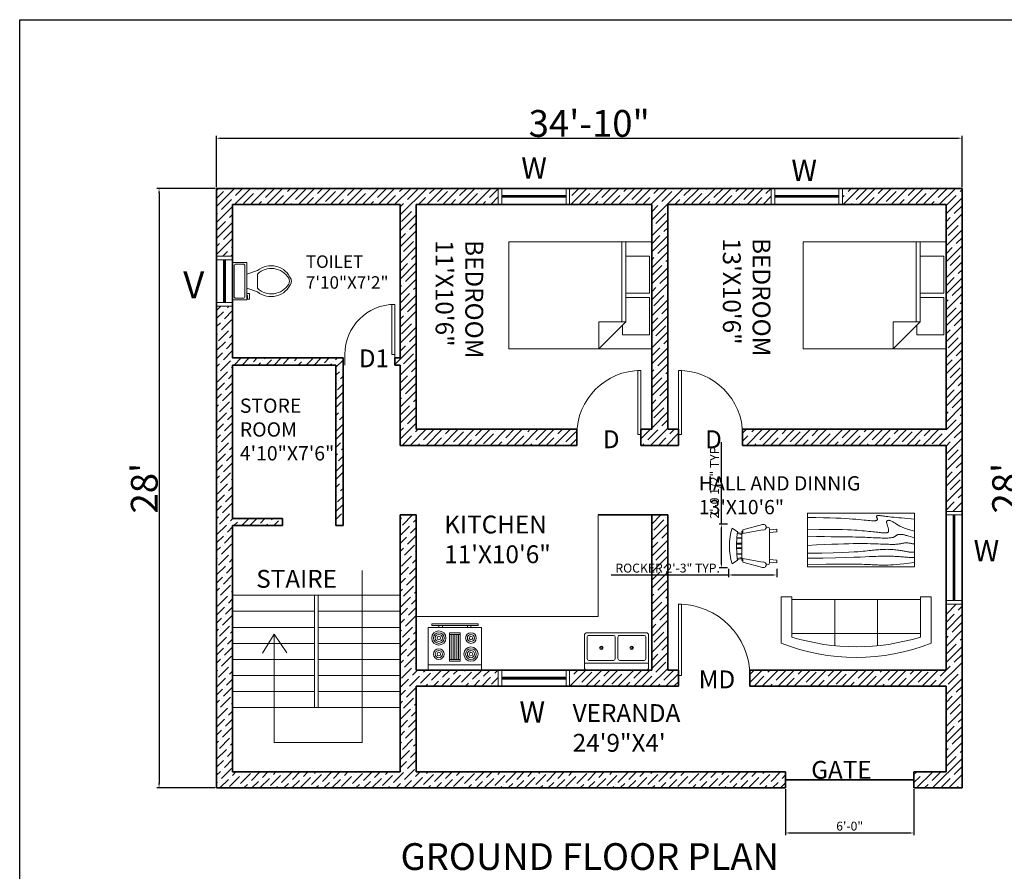
# Model space of a CAD drawing. Units: inches. Extents: x 1662 to 23131, y 1265 to 19127.
# Tile 12 of 26: x 17165 to 17717, y 8255 to 8732. Entities that reach past the tile are written whole.
import ezdxf

# ---------------------------------------------------------------- set-up
doc = ezdxf.new("R2010")
doc.units = ezdxf.units.IN
for name, color, linetype, lineweight in [('A-ANNO-DIMS', 4, 'Continuous', 18), ('A-ANNO-IDEN', 7, 'Continuous', 18), ('A-ANNO-TITL', 7, 'Continuous', 35), ('A-ANNO-TTLB', 7, 'Continuous', 25), ('A-AREA-IDEN', 7, 'Continuous', 18), ('A-DOOR', 3, 'Continuous', 18), ('A-EQPM', 8, 'Continuous', 18), ('A-FLOR-CASE', 8, 'Continuous', 18), ('A-FLOR-FIXT', 9, 'Continuous', 18), ('A-FLOR-STRS', 7, 'Continuous', 18), ('A-FURN', 8, 'Continuous', 18), ('A-GLAZ', 4, 'Continuous', 18), ('A-WALL', 7, 'Continuous', 35), ('A-WALL-PATT', 8, 'Continuous', 13)]:
    doc.layers.add(name, color=color, linetype=linetype, lineweight=lineweight)
doc.styles.get("Standard").update_dxf_attribs({"font": 'arial.ttf'})
doc.dimstyles.new('ISO-25', dxfattribs={"dimtxt": 5, "dimasz": 2.5, "dimexe": 1.25, "dimexo": 0.625, "dimtad": 1, "dimlunit": 3, "dimtxsty": 'Standard', "dimcen": 2.5, "dimadec": 0, "dimazin": 0, "dimtfac": 1, "dimtmove": 0, "dimatfit": 3, "dimfxl": 1, "dimarcsym": 0})

# ---------------------------------------------------------------- blocks, each defined once
blk = doc.blocks.new('*D63')
at = {"layer": 'A-ANNO-DIMS', "color": 0, "lineweight": -2, "transparency": 16777216}
for p, q in [((17275.26, 8638.02), (17275.26, 8666.76)), ((17693.26, 8638.02), (17693.26, 8666.76)), ((17277.76, 8665.51), (17690.76, 8665.51))]:
    blk.add_line(p, q, dxfattribs=at)
at = {"layer": 'A-ANNO-DIMS', "color": 0, "transparency": 16777216}
for points in [[(17277.76, 8665.93), (17277.76, 8665.09), (17275.26, 8665.51)], [(17690.76, 8665.93), (17690.76, 8665.09), (17693.26, 8665.51)]]:
    blk.add_solid(points, dxfattribs=at)
at = {"layer": 'Defpoints', "color": 0, "transparency": 16777216}
for p in [(17693.26, 8665.51), (17275.26, 8637.39), (17693.26, 8637.39)]:
    blk.add_point(p, dxfattribs=at)
at = {"layer": 'A-ANNO-DIMS', "color": 0, "transparency": 16777216, "insert": (17484.26, 8673.8), "char_height": 5, "attachment_point": 5}
blk.add_mtext('{\\H3x;34\'-10"}', dxfattribs=at)
blk = doc.blocks.new('*D64')
at = {"layer": 'A-ANNO-DIMS', "color": 0, "lineweight": -2, "transparency": 16777216}
for p, q in [((17274.63, 8637.39), (17241.85, 8637.39)), ((17243.1, 8634.89), (17243.1, 8303.89)), ((17274.63, 8301.39), (17241.85, 8301.39))]:
    blk.add_line(p, q, dxfattribs=at)
at = {"layer": 'A-ANNO-DIMS', "color": 0, "transparency": 16777216}
for points in [[(17242.68, 8634.89), (17243.51, 8634.89), (17243.1, 8637.39)], [(17242.68, 8303.89), (17243.51, 8303.89), (17243.1, 8301.39)]]:
    blk.add_solid(points, dxfattribs=at)
at = {"layer": 'Defpoints', "color": 0, "transparency": 16777216}
for p in [(17275.26, 8637.39), (17243.1, 8301.39), (17275.26, 8301.39)]:
    blk.add_point(p, dxfattribs=at)
at = {"layer": 'A-ANNO-DIMS', "color": 0, "transparency": 16777216, "insert": (17234.81, 8469.39), "char_height": 5, "attachment_point": 5, "rotation": 90}
blk.add_mtext("{\\H3x;28'}", dxfattribs=at)
blk = doc.blocks.new('*U10')
for p, q in [((0, 0), (0, -6)), ((40, 0), (40, -6))]:
    blk.add_line(p, q)
blk.add_lwpolyline([(0, 0), (0, 40), (1.75, 40), (1.75, 0)], close=True)
blk.add_arc((0, 0), 40, 0, 90)
blk = doc.blocks.new('*U67')
for p, q in [((0, 0), (0, -6)), ((36, 0), (36, -6))]:
    blk.add_line(p, q)
blk.add_lwpolyline([(0, 0), (0, 36), (1.75, 36), (1.75, 0)], close=True)
blk.add_arc((0, 0), 36, 0, 90)
blk = doc.blocks.new('*U34')
for p, q in [((0, 0), (0, -6)), ((-36, 0), (-36, -6))]:
    blk.add_line(p, q)
blk.add_lwpolyline([(0, 0), (0, 36), (-1.75, 36), (-1.75, 0)], close=True)
blk.add_arc((0, 0), 36, 90, 180)
blk = doc.blocks.new('*U68')
for p, q in [((-28, 0), (-28, -6)), ((0, 0), (0, -6))]:
    blk.add_line(p, q)
blk.add_lwpolyline([(0, 0), (0, 28), (-1.75, 28), (-1.75, 0)], close=True)
blk.add_arc((0, 0), 28, 90, 180)
blk = doc.blocks.new('Bed - Queen')
for p, q in [((0, -80.00003), (0, 0)), ((0, 0), (59.99999, 0)), ((59.99999, 0), (59.99999, -80.00003)), ((7.99999, -1.2), (28.79998, -1.2)), ((7.99999, -14.4), (7.99999, -1.2)), ((28.79998, -1.2), (28.79998, -14.4)), ((31.19999, -1.2), (51.99999, -1.2)), ((31.19999, -14.4), (31.19999, -1.2)), ((51.99999, -1.2), (51.99999, -16.4)), ((0, -14.4), (44.8, -14.4)), ((59.99999, -29.6), (44.8, -14.4)), ((44.8, -14.4), (44.8, -29.6)), ((51.99999, -16.4), (46.79936, -16.4)), ((44.8, -16.8), (0, -16.8)), ((44.8, -29.6), (59.99999, -29.6)), ((59.99999, -80.00003), (0, -80.00003))]:
    blk.add_line(p, q)
blk = doc.blocks.new('Toilet - top')
for p, q in [((9.5, -6), (9.5, -2)), ((-10, -8.5), (-8, -8.5)), ((-10, -9.5), (-10, -8.5)), ((-7, -9.5), (-10, -9.5)), ((-8, -8.5), (-8, -8)), ((-7, -8), (-7, -9.5)), ((-4, -8), (-6, -14)), ((4, -8), (6, -14)), ((4, -14), (-4, -14))]:
    blk.add_line(p, q)
blk.add_lwpolyline([(10.5, -8), (10.5, 0), (-10.5, 0), (-10.5, -8)], close=True)
for points in [[(-9.5, -2), (-9.5, -6)], [(8.5, -1), (-8.5, -1)], [(-8.5, -7), (8.5, -7)]]:
    blk.add_lwpolyline(points)
for centre, radius, start, end in [((-8.62, -1.88), 0.884, 81.8699, 188.1301), ((8.62, -1.88), 0.884, 351.8699, 98.1301), ((-8.62, -6.12), 0.884, 171.8699, 278.1301), ((8.62, -6.12), 0.884, 261.8699, 8.1301), ((3.52, -21.58), 12.17, 141.4691, 247.9714), ((4.2, -21.82), 11.33, 136.3677, 238.9468), ((-3.52, -21.58), 12.17, 292.0284, 38.5307), ((-4.2, -21.82), 11.33, 301.053, 43.6321), ((0, -27.88), 4, 245.7318, 294.2682), ((0, -29), 4, 254.8605, 285.1395)]:
    blk.add_arc(centre, radius, start, end)
blk = doc.blocks.new('Range-Oven - 30 in top')
for p, q in [((0, -3), (30, -3)), ((12, -6), (18, -6)), ((13, -20), (13, -6)), ((14, -6), (14, -20)), ((15, -20), (15, -6)), ((16, -6), (16, -20)), ((17, -20), (17, -6)), ((18, -20), (12, -20)), ((6, -24), (6, -25)), ((8, -25), (8, -24)), ((22, -25), (22, -24)), ((24, -24), (24, -25))]:
    blk.add_line(p, q)
for points in [[(0, -24), (0, 0), (30, 0), (30, -24)], [(12, -21), (12, -5), (18, -5), (18, -21)], [(2, -26), (2, -25), (28, -25), (28, -26)]]:
    blk.add_lwpolyline(points, close=True)
for centre, radius in [((6, -9), 4), ((6, -9), 3), ((6, -9), 2), ((6, -9), 1), ((24, -9), 3), ((24, -9), 2), ((24, -9), 1), ((6, -18), 3), ((6, -18), 2), ((24, -18), 4), ((24, -18), 3), ((24, -18), 2), ((6, -18), 1), ((24, -18), 1)]:
    blk.add_circle(centre, radius)
blk = doc.blocks.new('Sink-double - 36 in top')
for p, q in [((-18, -4), (18, -4)), ((-0.75, -18.5), (-0.75, -6.5)), ((0.75, -6.5), (0.75, -18.5))]:
    blk.add_line(p, q)
for points in [[(-16.5, 0), (16.5, 0)], [(-18, -19.5), (-18, -1.5)], [(-15.5, -5.5), (-1.75, -5.5)], [(1.75, -5.5), (15.5, -5.5)], [(18, -1.5), (18, -19.5)], [(-16.5, -18.5), (-16.5, -6.5)], [(16.5, -6.5), (16.5, -18.5)], [(16.5, -21), (-16.5, -21)], [(-1.75, -19.5), (-15.5, -19.5)], [(15.5, -19.5), (1.75, -19.5)]]:
    blk.add_lwpolyline(points)
for centre, radius in [((-8.5, -12.5), 1), ((-8.5, -12.5), 0.5), ((8.5, -12.5), 1), ((8.5, -12.5), 0.5)]:
    blk.add_circle(centre, radius)
for centre, radius, start, end in [((-16.5, -1.5), 1.5, 90, 180), ((16.5, -1.5), 1.5, 0, 90), ((-15.5, -6.5), 1, 90, 180), ((-1.75, -6.5), 1, 0, 90), ((1.75, -6.5), 1, 90, 180), ((15.5, -6.5), 1, 0, 90), ((-16.5, -19.5), 1.5, 180, 270), ((-15.5, -18.5), 1, 180, 270), ((-1.75, -18.5), 1, 270, 0), ((1.75, -18.5), 1, 180, 270), ((15.5, -18.5), 1, 270, 0), ((16.5, -19.5), 1.5, 270, 0)]:
    blk.add_arc(centre, radius, start, end)
blk = doc.blocks.new('Sofa - Roundback 7 ft.')
for p, q in [((-12.00002, -32.4421), (-12.00003, -6.5971)), ((11.99997, -32.4421), (11.99998, -6.5971)), ((-36.000027, -34), (-36.000027, -11.4696)), ((-35.999844, -13.3819), (35.9998, -13.3819)), ((35.99998, -34), (35.99998, -11.4696)), ((-36.000027, -32.4421), (35.99998, -32.4421))]:
    blk.add_line(p, q)
for points in [[(-36.000027, -34), (-42.000027, -34), (-42.000027, -8)], [(41.99998, -8), (41.99998, -34), (35.99998, -34)]]:
    blk.add_lwpolyline(points)
for centre, radius, start, end in [((0, -114.25), 114.25, 68.43141, 111.5686), ((-0.00001, -127.1968), 121.1968, 72.72033, 107.2797)]:
    blk.add_arc(centre, radius, start, end)
blk = doc.blocks.new('Table - Rectangular Woodgrain 60 x 30 in.')
for p, q in [((0, 0), (0, -30)), ((60, 0), (0, 0)), ((60, -30), (60, 0)), ((0, -30), (60, -30))]:
    blk.add_line(p, q)
for points in [[(0, -2.4), (4.8155, -2.418), (9.0302, -2.4688), (12.709, -2.5477), (15.9167, -2.65), (18.7181, -2.7711), (21.1781, -2.9063), (23.3616, -3.0508), (25.3333, -3.2), (27.1477, -3.3495), (28.8172, -3.4958), (30.3437, -3.636), (31.7291, -3.7667), (32.9756, -3.8849), (34.0849, -3.9875), (35.059, -4.0714), (35.9, -4.1334), (36.6114, -4.1711), (37.2041, -4.1854), (37.6906, -4.1779), (38.0833, -4.15), (38.3948, -4.1034), (38.6375, -4.0396), (38.8239, -3.9602), (38.9666, -3.8667), (39.0764, -3.7608), (39.1573, -3.6448), (39.2116, -3.521), (39.2416, -3.3917), (39.2498, -3.2593), (39.2385, -3.1261), (39.21, -2.9944), (39.1666, -2.8667), (39.111, -2.7447), (39.0468, -2.6281), (38.978, -2.5163), (38.9083, -2.4083), (38.8418, -2.3035), (38.7823, -2.201), (38.7337, -2.1001), (38.7, -2), (38.6844, -1.9003), (38.6875, -1.8021), (38.7094, -1.707), (38.75, -1.6167), (38.8094, -1.5326), (38.8875, -1.4563), (38.9844, -1.3893), (39.1, -1.3333), (39.2351, -1.2896), (39.3937, -1.2583), (39.5804, -1.2396), (39.8, -1.2333), (40.057, -1.2396), (40.3562, -1.2583), (40.7023, -1.2896), (41.1, -1.3333), (41.5547, -1.3895), (42.0755, -1.4573), (42.6721, -1.5361), (43.3542, -1.625), (44.1316, -1.7233), (45.014, -1.8302), (46.0114, -1.9449), (47.1333, -2.0667), (48.3862, -2.1947), (49.7625, -2.3281), (51.2513, -2.4663), (52.8416, -2.6083), (54.5226, -2.7535), (56.2833, -2.9011), (58.1127, -3.0501), (60, -3.2)], [(0, -9.2), (6.5759, -9.0858), (11.9385, -9.0365), (16.2527, -9.0418), (19.6833, -9.0917), (22.3952, -9.1759), (24.5531, -9.2844), (26.322, -9.4069), (27.8666, -9.5333), (29.3241, -9.6553), (30.7203, -9.7719), (32.0532, -9.8837), (33.3208, -9.9917), (34.5213, -10.0965), (35.6526, -10.199), (36.7128, -10.2999), (37.7, -10.4), (38.6129, -10.4996), (39.4531, -10.5969), (40.223, -10.6895), (40.925, -10.775), (41.5613, -10.8512), (42.1344, -10.9156), (42.6465, -10.966), (43.1, -11), (43.4976, -11.0158), (43.8437, -11.0136), (44.143, -10.9942), (44.4, -10.9583), (44.6195, -10.9069), (44.8062, -10.8406), (44.9648, -10.7603), (45.1, -10.6667), (45.2155, -10.5598), (45.3114, -10.4365), (45.3871, -10.2929), (45.4416, -10.125), (45.4743, -9.929), (45.4844, -9.7011), (45.4709, -9.4371), (45.4333, -9.1333), (45.3716, -8.7883), (45.2896, -8.4104), (45.1919, -8.0107), (45.0833, -7.6), (44.9685, -7.1893), (44.8521, -6.7896), (44.7388, -6.4117), (44.6333, -6.0667), (44.54, -5.7628), (44.4614, -5.4979), (44.4001, -5.2675), (44.3583, -5.0667), (44.3384, -4.8909), (44.3427, -4.7354), (44.3736, -4.5956), (44.4333, -4.4667), (44.5236, -4.3453), (44.6427, -4.2333), (44.7884, -4.1339), (44.9583, -4.05), (45.1501, -3.9849), (45.3614, -3.9417), (45.59, -3.9234), (45.8333, -3.9333), (46.0915, -3.9749), (46.3734, -4.0531), (46.6906, -4.1736), (47.0542, -4.3417), (47.4756, -4.5629), (47.9661, -4.8427), (48.5372, -5.1866), (49.2, -5.6), (49.9676, -6.0844), (50.8594, -6.625), (51.8965, -7.2031), (53.1, -7.8), (54.491, -8.3969), (56.0906, -8.975), (57.9199, -9.5156), (60, -10)], [(0, -12.8), (5.1847, -12.9322), (9.6213, -13.0323), (13.3963, -13.1059), (16.5958, -13.1583), (19.3063, -13.1952), (21.614, -13.2219), (23.6054, -13.2439), (25.3666, -13.2667), (26.9728, -13.2947), (28.4531, -13.3281), (29.8256, -13.3663), (31.1083, -13.4083), (32.3191, -13.4535), (33.476, -13.501), (34.597, -13.5501), (35.7, -13.6), (36.7984, -13.6497), (37.8875, -13.6979), (38.9578, -13.743), (40, -13.7833), (41.0047, -13.8174), (41.9625, -13.8438), (42.864, -13.8607), (43.7, -13.8667), (44.4631, -13.8604), (45.1552, -13.8417), (45.7801, -13.8104), (46.3416, -13.7667), (46.8439, -13.7104), (47.2906, -13.6417), (47.6858, -13.5604), (48.0333, -13.4667), (48.3375, -13.3608), (48.6042, -13.2448), (48.8396, -13.121), (49.05, -12.9917), (49.2417, -12.8593), (49.4208, -12.7261), (49.5937, -12.5944), (49.7667, -12.4667), (49.9452, -12.3451), (50.1323, -12.2313), (50.3303, -12.1268), (50.5416, -12.0333), (50.7686, -11.9524), (51.0135, -11.8854), (51.2788, -11.8341), (51.5666, -11.8), (51.8785, -11.7843), (52.2116, -11.7865), (52.562, -11.8059), (52.926, -11.8417), (53.2998, -11.8931), (53.6795, -11.9594), (54.0614, -12.0397), (54.4416, -12.1333), (54.8223, -12.2401), (55.2293, -12.3625), (55.6942, -12.5037), (56.2489, -12.6667), (56.9251, -12.8547), (57.7545, -13.0708), (58.7689, -13.3182), (60, -13.6)], [(0, -18), (5.124, -17.7273), (9.6609, -17.5057), (13.6705, -17.3303), (17.2125, -17.1958), (20.3467, -17.0973), (23.1328, -17.0297), (25.6307, -16.9878), (27.9, -16.9667), (29.9928, -16.9617), (31.9302, -16.9703), (33.7254, -16.9907), (35.3917, -17.0208), (36.9423, -17.0588), (38.3906, -17.1026), (39.7499, -17.1503), (41.0333, -17.2), (42.2519, -17.2496), (43.4073, -17.2969), (44.4986, -17.3395), (45.525, -17.375), (46.4858, -17.4012), (47.3802, -17.4156), (48.2074, -17.416), (48.9667, -17.4), (49.6583, -17.3662), (50.2872, -17.3167), (50.8595, -17.2547), (51.3812, -17.1833), (51.8584, -17.1057), (52.2971, -17.025), (52.7034, -16.9443), (53.0833, -16.8667), (53.443, -16.7951), (53.789, -16.7313), (54.128, -16.6768), (54.4666, -16.6334), (54.8115, -16.6024), (55.1693, -16.5854), (55.5465, -16.5841), (55.95, -16.6), (56.3828, -16.6337), (56.8346, -16.6823), (57.2915, -16.7418), (57.7396, -16.8084), (58.165, -16.878), (58.5539, -16.9469), (58.8924, -17.0111), (59.1666, -17.0667), (59.3679, -17.1107), (59.5078, -17.1438), (59.6032, -17.1675), (59.6708, -17.1833), (59.7275, -17.193), (59.7901, -17.1979), (59.8753, -17.1998), (60, -17.2)], [(0, -22.4), (8.0098, -22.2501), (14.4094, -22.1011), (19.4168, -21.9535), (23.25, -21.8083), (26.1269, -21.6663), (28.2656, -21.5281), (29.884, -21.3947), (31.2, -21.2667), (32.3967, -21.1448), (33.5172, -21.0292), (34.5697, -20.9198), (35.5625, -20.8167), (36.5037, -20.7198), (37.4015, -20.6292), (38.2642, -20.5448), (39.1, -20.4667), (39.9164, -20.3951), (40.7187, -20.3313), (41.5117, -20.2768), (42.3, -20.2333), (43.0883, -20.2024), (43.8812, -20.1854), (44.6836, -20.1841), (45.5, -20.2), (46.3328, -20.234), (47.1747, -20.2844), (48.0163, -20.3488), (48.8479, -20.425), (49.66, -20.5106), (50.4429, -20.6031), (51.1872, -20.7004), (51.8833, -20.8), (52.5246, -20.8999), (53.1166, -20.9995), (53.6681, -21.0983), (54.1875, -21.1958), (54.6834, -21.2919), (55.1646, -21.3859), (55.6394, -21.4777), (56.1167, -21.5667), (56.6028, -21.6515), (57.0961, -21.7266), (57.5929, -21.7852), (58.0896, -21.8208), (58.5823, -21.8268), (59.0674, -21.7964), (59.5412, -21.723), (60, -21.6)], [(0, -25.2), (8.6355, -25.0504), (15.7026, -24.9031), (21.4049, -24.7606), (25.9458, -24.625), (29.529, -24.4988), (32.3578, -24.3844), (34.6359, -24.284), (36.5667, -24.2), (38.3213, -24.1341), (39.9417, -24.0854), (41.437, -24.0523), (42.8167, -24.0333), (44.0901, -24.0268), (45.2667, -24.0313), (46.3557, -24.0451), (47.3667, -24.0667), (48.309, -24.0947), (49.1928, -24.1287), (50.0284, -24.168), (50.826, -24.2125), (51.5959, -24.2617), (52.3483, -24.3151), (53.0935, -24.3725), (53.8417, -24.4334), (54.6009, -24.497), (55.3699, -24.561), (56.1454, -24.6226), (56.9239, -24.6792), (57.7021, -24.7279), (58.4764, -24.7662), (59.2435, -24.7911), (60, -24.8)], [(0, -28.8), (5.6867, -28.6681), (10.45, -28.5698), (14.407, -28.5012), (17.675, -28.4584), (20.3711, -28.4374), (22.6125, -28.4344), (24.5164, -28.4455), (26.2, -28.4667), (27.762, -28.4947), (29.2276, -28.5281), (30.6033, -28.5663), (31.8958, -28.6084), (33.1118, -28.6535), (34.2578, -28.7011), (35.3405, -28.7501), (36.3666, -28.8), (37.3443, -28.8497), (38.288, -28.8974), (39.2137, -28.9412), (40.1375, -28.9792), (41.0753, -29.0093), (42.0432, -29.0297), (43.0572, -29.0384), (44.1333, -29.0333), (45.2936, -29.0114), (46.5843, -28.9641), (48.0579, -28.8816), (49.7666, -28.7542), (51.7629, -28.5721), (54.0989, -28.3255), (56.8272, -28.0048), (60, -27.6)]]:
    blk.add_lwpolyline(points)
blk = doc.blocks.new('Chair - Rocking')
for p, q in [((-8, -4.5), (-10, -1.5)), ((-7.5, -4.5), (-7, -7)), ((-6.5, -7), (-7.02225, -4.43)), ((-4.5, -7), (-4.96674, -4.19951)), ((-4, -7), (-4.40532, -4.16272)), ((-1.5, -4.05012), (-1.5, -7)), ((-1, -7), (-1, -4.05012)), ((1, -7), (1, -4.04655)), ((1.5, -4.05012), (1.5, -7)), ((4, -7), (4.40187, -4.18694)), ((4.5, -7), (4.96761, -4.19437)), ((6.5, -7), (7, -4.4057)), ((7.5, -4.5), (7, -7)), ((8, -4.5), (10, -1.5)), ((-9, -7.5), (-12, -18.49999)), ((-7, -7.5), (-9, -7.5)), ((-9, -18.49999), (-7, -7.5)), ((-8.23428, -6.99939), (-8.3093, -7.47958)), ((-8.23041, -7), (8.23915, -7)), ((7, -7.5), (9, -7.5)), ((9, -18.49999), (7, -7.5)), ((8.31071, -7.48854), (8.23449, -7.00073)), ((9, -7.5), (12, -18.49999)), ((-10.36644, -20.64523), (-10.5, -21.49999)), ((10.5, -21.49999), (10.3575, -20.58798)), ((-9, -22.49999), (-9.5, -26.49999)), ((0, -22.49999), (-9.5, -22.49999)), ((-9.5, -26.49999), (-8, -26.49999)), ((-8, -26.49999), (-7.5, -22.49999)), ((0, -22.49999), (9.5, -22.49999)), ((8, -26.49999), (7.5, -22.49999)), ((9.5, -26.49999), (8, -26.49999)), ((9, -22.49999), (9.5, -26.49999))]:
    blk.add_line(p, q)
for centre, radius, start, end in [((0, -34.08333), 34.08333, 72.93847, 107.0615), ((0, -68.25004), 64.25, 93.92211, 97.15267), ((0, -68.25004), 64.25, 82.84733, 93.92211), ((-10.5, -18.99999), 1.58114, 161.5651, 18.43495), ((-9.5, -21.49999), 1, 180, 270), ((10.5, -18.99999), 1.58114, 161.5651, 18.43495), ((9.5, -21.49999), 1, 270, 0)]:
    blk.add_arc(centre, radius, start, end)
blk = doc.blocks.new('*D74')
at = {"layer": 'A-ANNO-DIMS', "color": 0, "lineweight": -2, "transparency": 16777216}
for p, q in [((17756.47, 8637.39), (17724.69, 8637.39)), ((17725.94, 8634.89), (17725.94, 8303.89)), ((17756.47, 8301.39), (17724.69, 8301.39))]:
    blk.add_line(p, q, dxfattribs=at)
at = {"layer": 'A-ANNO-DIMS', "color": 0, "transparency": 16777216}
for points in [[(17725.53, 8634.89), (17726.36, 8634.89), (17725.94, 8637.39)], [(17725.53, 8303.89), (17726.36, 8303.89), (17725.94, 8301.39)]]:
    blk.add_solid(points, dxfattribs=at)
at = {"layer": 'Defpoints', "color": 0, "transparency": 16777216}
for p in [(17757.09, 8637.39), (17725.94, 8301.39), (17757.09, 8301.39)]:
    blk.add_point(p, dxfattribs=at)
at = {"layer": 'A-ANNO-DIMS', "color": 0, "transparency": 16777216, "insert": (17717.66, 8469.39), "char_height": 5, "attachment_point": 5, "rotation": 90}
blk.add_mtext("{\\H3x;28'}", dxfattribs=at)
blk = doc.blocks.new('*D179')
at = {"layer": 'A-ANNO-DIMS', "color": 0, "lineweight": -2, "transparency": 16777216}
for p, q in [((17562.37, 8424.15), (17562.37, 8419.47)), ((17589.37, 8424.15), (17589.37, 8419.47)), ((17562.37, 8420.72), (17496.58, 8420.72)), ((17586.87, 8420.72), (17564.87, 8420.72))]:
    blk.add_line(p, q, dxfattribs=at)
at = {"layer": 'A-ANNO-DIMS', "color": 0, "transparency": 16777216}
for points in [[(17564.87, 8421.14), (17564.87, 8420.31), (17562.37, 8420.72)], [(17586.87, 8421.14), (17586.87, 8420.31), (17589.37, 8420.72)]]:
    blk.add_solid(points, dxfattribs=at)
at = {"layer": 'Defpoints', "color": 0, "transparency": 16777216}
for p in [(17562.37, 8424.77), (17589.37, 8424.77), (17562.37, 8420.72)]:
    blk.add_point(p, dxfattribs=at)
at = {"layer": 'A-ANNO-DIMS', "color": 0, "transparency": 16777216, "insert": (17528.22, 8423.94), "char_height": 5, "attachment_point": 5}
blk.add_mtext('ROCKER 2\'-3" TYP.', dxfattribs=at)
blk = doc.blocks.new('*D180')
at = {"layer": 'A-ANNO-DIMS', "color": 0, "lineweight": -2, "transparency": 16777216}
for p, q in [((17558.32, 8449.21), (17558.32, 8495.17)), ((17561.74, 8449.21), (17557.07, 8449.21)), ((17558.32, 8427.27), (17558.32, 8446.71)), ((17561.74, 8424.77), (17557.07, 8424.77))]:
    blk.add_line(p, q, dxfattribs=at)
at = {"layer": 'A-ANNO-DIMS', "color": 0, "transparency": 16777216}
for points in [[(17557.9, 8446.71), (17558.74, 8446.71), (17558.32, 8449.21)], [(17557.9, 8427.27), (17558.74, 8427.27), (17558.32, 8424.77)]]:
    blk.add_solid(points, dxfattribs=at)
at = {"layer": 'Defpoints', "color": 0, "transparency": 16777216}
for p in [(17558.32, 8449.21), (17562.37, 8449.21), (17562.37, 8424.77)]:
    blk.add_point(p, dxfattribs=at)
at = {"layer": 'A-ANNO-DIMS', "color": 0, "transparency": 16777216, "insert": (17555.11, 8473.44), "char_height": 5, "attachment_point": 5, "rotation": 90}
blk.add_mtext('2\'-0 1/2" TYP.', dxfattribs=at)
blk = doc.blocks.new('*D228')
at = {"layer": 'A-ANNO-DIMS', "color": 0, "lineweight": -2, "transparency": 16777216}
for p, q in [((17594.26, 8300.77), (17594.26, 8274.89)), ((17666.26, 8300.77), (17666.26, 8274.89)), ((17596.76, 8276.14), (17663.76, 8276.14))]:
    blk.add_line(p, q, dxfattribs=at)
at = {"layer": 'A-ANNO-DIMS', "color": 0, "transparency": 16777216}
for points in [[(17596.76, 8276.56), (17596.76, 8275.73), (17594.26, 8276.14)], [(17663.76, 8276.56), (17663.76, 8275.73), (17666.26, 8276.14)]]:
    blk.add_solid(points, dxfattribs=at)
at = {"layer": 'Defpoints', "color": 0, "transparency": 16777216}
for p in [(17594.26, 8301.39), (17666.26, 8301.39), (17666.26, 8276.14)]:
    blk.add_point(p, dxfattribs=at)
at = {"layer": 'A-ANNO-DIMS', "color": 0, "transparency": 16777216, "insert": (17630.26, 8279.32), "char_height": 5, "attachment_point": 5}
blk.add_mtext('6\'-0"', dxfattribs=at)

msp = doc.modelspace()

# ---------------------------------------------------------------- hatches: boundary and pattern name
at = {"layer": 'A-WALL-PATT'}
h = msp.add_hatch(dxfattribs=at)
h.set_pattern_fill('ANSI35', color=256)
h.paths.add_polyline_path([(17275.258, 8599.392), (17284.258, 8599.392), (17284.258, 8628.392), (17378.258, 8628.392), (17378.258, 8542.392), (17375.258, 8542.392), (17375.258, 8538.392), (17378.258, 8538.392), (17378.258, 8493.392), (17477.258, 8493.392), (17477.258, 8502.392), (17387.258, 8502.392), (17387.258, 8628.392), (17433.258, 8628.392), (17433.258, 8637.392), (17275.258, 8637.392)])
h.paths.add_polyline_path([(17473.258, 8637.392), (17473.258, 8628.392), (17519.258, 8628.392), (17519.258, 8502.392), (17513.258, 8502.392), (17513.258, 8499.392), (17513.258, 8493.392), (17534.258, 8493.392), (17534.258, 8499.392), (17534.258, 8502.392), (17528.258, 8502.392), (17528.258, 8628.392), (17586.258, 8628.392), (17586.258, 8637.392)])
h.paths.add_polyline_path([(17626.258, 8637.392), (17626.258, 8628.392), (17684.258, 8628.392), (17684.258, 8502.392), (17570.258, 8502.392), (17570.258, 8493.392), (17684.258, 8493.392), (17684.258, 8456.392), (17693.258, 8456.392), (17693.258, 8637.392)])
h.paths.add_polyline_path([(17684.258, 8367.392), (17574.258, 8367.392), (17574.258, 8358.392), (17684.258, 8358.392), (17684.258, 8310.392), (17666.258, 8310.392), (17666.258, 8301.392), (17693.258, 8301.392), (17693.258, 8404.392), (17684.258, 8404.392)])
h.paths.add_polyline_path([(17534.258, 8358.392), (17534.258, 8364.392), (17534.258, 8367.392), (17528.258, 8367.392), (17528.258, 8454.392), (17519.258, 8454.392), (17519.258, 8367.392), (17473.258, 8367.392), (17473.258, 8358.392)])
h = msp.add_hatch(dxfattribs=at)
h.set_pattern_fill('ANSI36', color=256)
h.paths.add_polyline_path([(17284.258, 8538.392), (17342.258, 8538.392), (17342.258, 8448.392), (17346.258, 8448.392), (17346.258, 8542.392), (17284.258, 8542.392), (17284.258, 8571.392), (17275.258, 8571.392), (17275.258, 8301.392), (17594.258, 8301.392), (17594.258, 8310.392), (17387.258, 8310.392), (17387.258, 8358.392), (17433.258, 8358.392), (17433.258, 8367.392), (17387.258, 8367.392), (17387.258, 8454.392), (17378.258, 8454.392), (17378.258, 8310.392), (17284.258, 8310.392), (17284.258, 8448.392), (17312.258, 8448.392), (17312.258, 8452.392), (17284.258, 8452.392)])

# ---------------------------------------------------------------- linework, layer by layer
at = {"layer": 'A-ANNO-TTLB'}
msp.add_lwpolyline([(17164.976, 8731.935), (18265.142, 8731.935), (18265.142, 7742.121), (17164.976, 7742.121)], close=True, dxfattribs=at)
at = {"layer": 'A-FLOR-CASE'}
for p in [(17489.258, 8454.392), (17387.258, 8397.392)]:
    msp.add_line(p, (17489.258, 8397.392), dxfattribs=at)
at = {"layer": 'A-FLOR-STRS'}
for p, q in [((17356.925, 8423.308), (17356.925, 8326.864)), ((17378.258, 8409.392), (17284.258, 8409.392)), ((17330.258, 8346.392), (17330.258, 8409.392)), ((17332.258, 8346.392), (17332.258, 8409.392)), ((17330.258, 8400.392), (17284.258, 8400.392)), ((17378.258, 8400.392), (17332.258, 8400.392)), ((17330.258, 8391.392), (17284.258, 8391.392)), ((17378.258, 8391.392), (17332.258, 8391.392)), ((17307.661, 8387.615), (17301.101, 8376.998)), ((17307.661, 8326.864), (17307.661, 8387.615)), ((17307.661, 8387.615), (17314.825, 8377.167)), ((17330.258, 8382.392), (17284.258, 8382.392)), ((17378.258, 8382.392), (17332.258, 8382.392)), ((17330.258, 8373.392), (17284.258, 8373.392)), ((17378.258, 8373.392), (17332.258, 8373.392)), ((17330.258, 8364.392), (17284.258, 8364.392)), ((17378.258, 8364.392), (17332.258, 8364.392)), ((17330.258, 8355.392), (17284.258, 8355.392)), ((17378.258, 8355.392), (17332.258, 8355.392)), ((17378.258, 8346.392), (17284.258, 8346.392)), ((17356.925, 8326.864), (17307.661, 8326.864))]:
    msp.add_line(p, q, dxfattribs=at)
at = {"layer": 'A-GLAZ'}
for p, q in [((17433.258, 8628.392), (17433.258, 8637.392)), ((17435.258, 8628.392), (17435.258, 8637.392)), ((17471.258, 8633.392), (17435.258, 8633.392)), ((17471.258, 8632.892), (17435.258, 8632.892)), ((17471.258, 8628.392), (17471.258, 8637.392)), ((17473.258, 8628.392), (17473.258, 8637.392)), ((17586.258, 8628.392), (17586.258, 8637.392)), ((17588.258, 8628.392), (17588.258, 8637.392)), ((17624.258, 8633.392), (17588.258, 8633.392)), ((17624.258, 8632.892), (17588.258, 8632.892)), ((17624.258, 8628.392), (17624.258, 8637.392)), ((17626.258, 8628.392), (17626.258, 8637.392)), ((17471.258, 8632.392), (17435.258, 8632.392)), ((17624.258, 8632.392), (17588.258, 8632.392)), ((17284.258, 8599.392), (17275.258, 8599.392)), ((17284.258, 8597.392), (17275.258, 8597.392)), ((17279.258, 8597.392), (17279.258, 8573.392)), ((17279.758, 8597.392), (17279.758, 8573.392)), ((17280.258, 8597.392), (17280.258, 8573.392)), ((17284.258, 8573.392), (17275.258, 8573.392)), ((17284.258, 8571.392), (17275.258, 8571.392)), ((17693.258, 8456.392), (17684.258, 8456.392)), ((17693.258, 8454.392), (17684.258, 8454.392)), ((17688.258, 8454.392), (17688.258, 8406.392)), ((17688.758, 8454.392), (17688.758, 8406.392)), ((17689.258, 8454.392), (17689.258, 8406.392)), ((17693.258, 8406.392), (17684.258, 8406.392)), ((17693.258, 8404.392), (17684.258, 8404.392)), ((17433.258, 8358.392), (17433.258, 8367.392)), ((17435.258, 8358.392), (17435.258, 8367.392)), ((17471.258, 8363.392), (17435.258, 8363.392)), ((17471.258, 8362.892), (17435.258, 8362.892)), ((17471.258, 8362.392), (17435.258, 8362.392)), ((17471.258, 8358.392), (17471.258, 8367.392)), ((17473.258, 8358.392), (17473.258, 8367.392))]:
    msp.add_line(p, q, dxfattribs=at)
at = {"layer": 'A-WALL'}
for p, q in [((17275.258, 8637.392), (17693.258, 8637.392)), ((17275.258, 8301.392), (17275.258, 8637.392)), ((17693.258, 8637.392), (17693.258, 8301.392)), ((17284.258, 8628.392), (17378.258, 8628.392)), ((17284.258, 8542.392), (17284.258, 8628.392)), ((17378.258, 8628.392), (17378.258, 8542.392)), ((17387.258, 8628.392), (17387.258, 8502.392)), ((17387.258, 8628.392), (17519.258, 8628.392)), ((17519.258, 8628.392), (17519.258, 8502.392)), ((17528.258, 8628.392), (17528.258, 8502.392)), ((17528.258, 8628.392), (17684.258, 8628.392)), ((17684.258, 8628.392), (17684.258, 8502.392)), ((17284.258, 8542.392), (17346.258, 8542.392)), ((17346.258, 8542.392), (17346.258, 8448.392)), ((17375.258, 8542.392), (17375.258, 8538.392)), ((17375.258, 8542.392), (17378.258, 8542.392)), ((17284.258, 8538.392), (17342.258, 8538.392)), ((17284.258, 8452.392), (17284.258, 8538.392)), ((17342.258, 8538.392), (17342.258, 8448.392)), ((17375.258, 8538.392), (17378.258, 8538.392)), ((17378.258, 8538.392), (17378.258, 8493.392)), ((17387.258, 8502.392), (17477.258, 8502.392)), ((17477.258, 8502.392), (17477.258, 8493.392)), ((17513.258, 8502.392), (17513.258, 8493.392)), ((17513.258, 8502.392), (17519.258, 8502.392)), ((17528.258, 8502.392), (17534.258, 8502.392)), ((17534.258, 8502.392), (17534.258, 8493.392)), ((17570.258, 8502.392), (17570.258, 8493.392)), ((17570.258, 8502.392), (17684.258, 8502.392)), ((17378.258, 8493.392), (17477.258, 8493.392)), ((17513.258, 8493.392), (17534.258, 8493.392)), ((17570.258, 8493.392), (17684.258, 8493.392)), ((17684.258, 8493.392), (17684.258, 8367.392)), ((17284.258, 8452.392), (17312.258, 8452.392)), ((17312.258, 8452.392), (17312.258, 8448.392)), ((17378.258, 8454.392), (17378.258, 8310.392)), ((17378.258, 8454.392), (17387.258, 8454.392)), ((17387.258, 8454.392), (17387.258, 8367.392)), ((17489.258, 8454.392), (17528.258, 8454.392)), ((17519.258, 8454.392), (17519.258, 8367.392)), ((17528.258, 8454.392), (17528.258, 8367.392)), ((17284.258, 8310.392), (17284.258, 8448.392)), ((17284.258, 8448.392), (17312.258, 8448.392)), ((17342.258, 8448.392), (17346.258, 8448.392)), ((17387.258, 8367.392), (17519.258, 8367.392)), ((17528.258, 8367.392), (17534.258, 8367.392)), ((17534.258, 8367.392), (17534.258, 8358.392)), ((17574.258, 8367.392), (17574.258, 8358.392)), ((17574.258, 8367.392), (17684.258, 8367.392)), ((17387.258, 8358.392), (17534.258, 8358.392)), ((17387.258, 8358.392), (17387.258, 8310.392)), ((17574.258, 8358.392), (17684.258, 8358.392)), ((17684.258, 8358.392), (17684.258, 8310.392)), ((17378.258, 8310.392), (17284.258, 8310.392)), ((17594.258, 8310.392), (17387.258, 8310.392)), ((17594.258, 8310.392), (17594.258, 8301.392)), ((17684.258, 8310.392), (17666.258, 8310.392)), ((17666.258, 8310.392), (17666.258, 8301.392)), ((17594.258, 8305.892), (17666.258, 8305.892)), ((17594.258, 8301.392), (17275.258, 8301.392)), ((17693.258, 8301.392), (17666.258, 8301.392))]:
    msp.add_line(p, q, dxfattribs=at)

# ---------------------------------------------------------------- block references
at = {"layer": 'A-DOOR'}
for name, p in [('*U68', (17375.258, 8544.392)), ('*U34', (17513.258, 8499.392)), ('*U67', (17534.258, 8499.392)), ('*U10', (17534.258, 8364.392))]:
    msp.add_blockref(name, p, dxfattribs=at)
at = {"layer": 'A-EQPM', "rotation": 180}
msp.add_blockref('Range-Oven - 30 in top', (17423.941, 8367.392), dxfattribs=at)
at = {"layer": 'A-FLOR-FIXT'}
for name, p, rotation in [('Toilet - top', (17284.258, 8585.392), 90), ('Sink-double - 36 in top', (17499.57, 8367.392), 180)]:
    msp.add_blockref(name, p, dxfattribs=dict(at, rotation=rotation))
at = {"layer": 'A-FURN'}
for name, p, rotation in [('Bed - Queen', (17519.258, 8607.392), 270), ('Bed - Queen', (17684.258, 8607.392), 270), ('Chair - Rocking', (17562.87, 8436.99), 90), ('Sofa - Roundback 7 ft.', (17633.903, 8374.478), 180)]:
    msp.add_blockref(name, p, dxfattribs=dict(at, rotation=rotation))
msp.add_blockref('Table - Rectangular Woodgrain 60 x 30 in.', (17606.558, 8455.291), dxfattribs=at)

# ---------------------------------------------------------------- texts
at = {"layer": 'A-ANNO-IDEN', "attachment_point": 1}
for s, width, heights, insert, char_height in [('W', 471.52273, [28.462], (17446.153, 8654.851), 12), ('W', 471.52273, [28.462], (17597.556, 8653.577), 12), ('V', 1142.59551, [20], (17256.659, 8590.83), 15), ('D1', 1142.59551, [20], (17355.082, 8547.135), 10), ('D', 1142.59551, [0], (17491.866, 8501.787), 10), ('D', 1142.59551, [0], (17549.219, 8501.787), 10), ('W', 471.52273, [28.462], (17699.722, 8440.381), 12), ('MD', 1142.59551, [0], (17545.615, 8367.206), 10), ('W', 471.52273, [28.462], (17445.135, 8349.97), 12)]:
    msp.add_mtext_dynamic_manual_height_columns(s, width=width, gutter_width=12.5, heights=heights, dxfattribs=dict(at, insert=insert, char_height=char_height))
at = {"layer": 'A-ANNO-TITL', "insert": (17378.476, 8270.416), "char_height": 15, "attachment_point": 1}
msp.add_mtext_dynamic_manual_height_columns('GROUND FLOOR PLAN', width=1142.59551, gutter_width=12.5, heights=[0], dxfattribs=at)
at = {"layer": 'A-AREA-IDEN', "char_height": 10, "attachment_point": 1, "rotation": 270}
for s, insert in [('BEDROOM\\P11\'X10\'6"', (17424.809, 8608.438)), ('BEDROOM\\P13\'X10\'6"', (17585.86, 8609.566))]:
    msp.add_mtext_dynamic_manual_height_columns(s, width=1142.59551, gutter_width=12.5, heights=[277.772], dxfattribs=dict(at, insert=insert))
at = {"layer": 'A-AREA-IDEN', "attachment_point": 1}
for s, heights, insert, char_height in [('TOILET\\P7\'10"X7\'2"', [277.772], (17325.413, 8599.845), 7), ('STORE \\PROOM\\P4\'10"X7\'6"', [0], (17288.379, 8519.617), 8), ('HALL AND DINNIG\\P13\'X10\'6"', [277.772], (17545.686, 8476.102), 8), ('KITCHEN\\P11\'X10\'6"', [277.772], (17402.97, 8454.016), 10), ('STAIRE', [0], (17297.57, 8423.562), 10), ('VERANDA\\P24\'9"X4\'', [277.772], (17474.958, 8348.35), 10), ('GATE', [0], (17608.691, 8316.527), 10)]:
    msp.add_mtext_dynamic_manual_height_columns(s, width=1142.59551, gutter_width=12.5, heights=heights, dxfattribs=dict(at, insert=insert, char_height=char_height))

# ---------------------------------------------------------------- dimensions: what is measured, and where the dimension line sits
at = {"layer": 'A-ANNO-DIMS'}
dim = msp.add_linear_dim(base=(17693.258, 8665.51), p1=(17275.258, 8637.392), p2=(17693.258, 8637.392), text='{\\H3x;<>}', dimstyle='ISO-25', override={"dimclrd": 0, "dimclre": 0, "dimclrt": 0}, dxfattribs=at)
dim.commit()
dim.dimension.update_dxf_attribs({"geometry": '*D63', "text_midpoint": (17484.258, 8673.799)})
for base, p1, p2, angle, text, override, picture, middle in [((17243.097, 8301.392), (17275.258, 8637.392), (17275.258, 8301.392), 90, '{\\H3x;<>}', {"dimclrd": 0, "dimclre": 0, "dimclrt": 0}, '*D64', (17234.814, 8469.392)), ((17725.942, 8301.392), (17757.093, 8637.392), (17757.093, 8301.392), 90, '{\\H3x;<>}', {"dimclrd": 0, "dimclre": 0, "dimclrt": 0}, '*D74', (17717.658, 8469.392)), ((17558.32, 8449.207), (17562.37, 8424.772), (17562.37, 8449.207), 90, '<> TYP.', {"dimdec": 1, "dimlfac": 1, "dimrnd": 0, "dimzin": 1, "dimdsep": 46, "dimlunit": 4, "dimfrac": 2}, '*D180', (17555.11, 8473.439)), ((17562.37, 8420.722), (17589.37, 8424.772), (17562.37, 8424.772), 180, 'ROCKER <> TYP.', {"dimdec": 1, "dimlfac": 1, "dimrnd": 0, "dimzin": 1, "dimdsep": 46, "dimlunit": 4, "dimfrac": 2}, '*D179', (17528.223, 8423.936))]:
    dim = msp.add_linear_dim(base=base, p1=p1, p2=p2, angle=angle, text=text, dimstyle='ISO-25', override=override, dxfattribs=at)
    dim.commit()
    dim.dimension.update_dxf_attribs({"geometry": picture, "text_midpoint": middle})
dim = msp.add_linear_dim(base=(17666.258, 8276.142), p1=(17594.258, 8301.392), p2=(17666.258, 8301.392), dimstyle='ISO-25', override={"dimdec": 1, "dimlfac": 1, "dimrnd": 0, "dimzin": 1, "dimdsep": 46, "dimlunit": 4, "dimfrac": 2}, dxfattribs=at)
dim.commit()
dim.dimension.update_dxf_attribs({"geometry": '*D228', "text_midpoint": (17630.258, 8279.32)})

doc.saveas('drawing.dxf')
